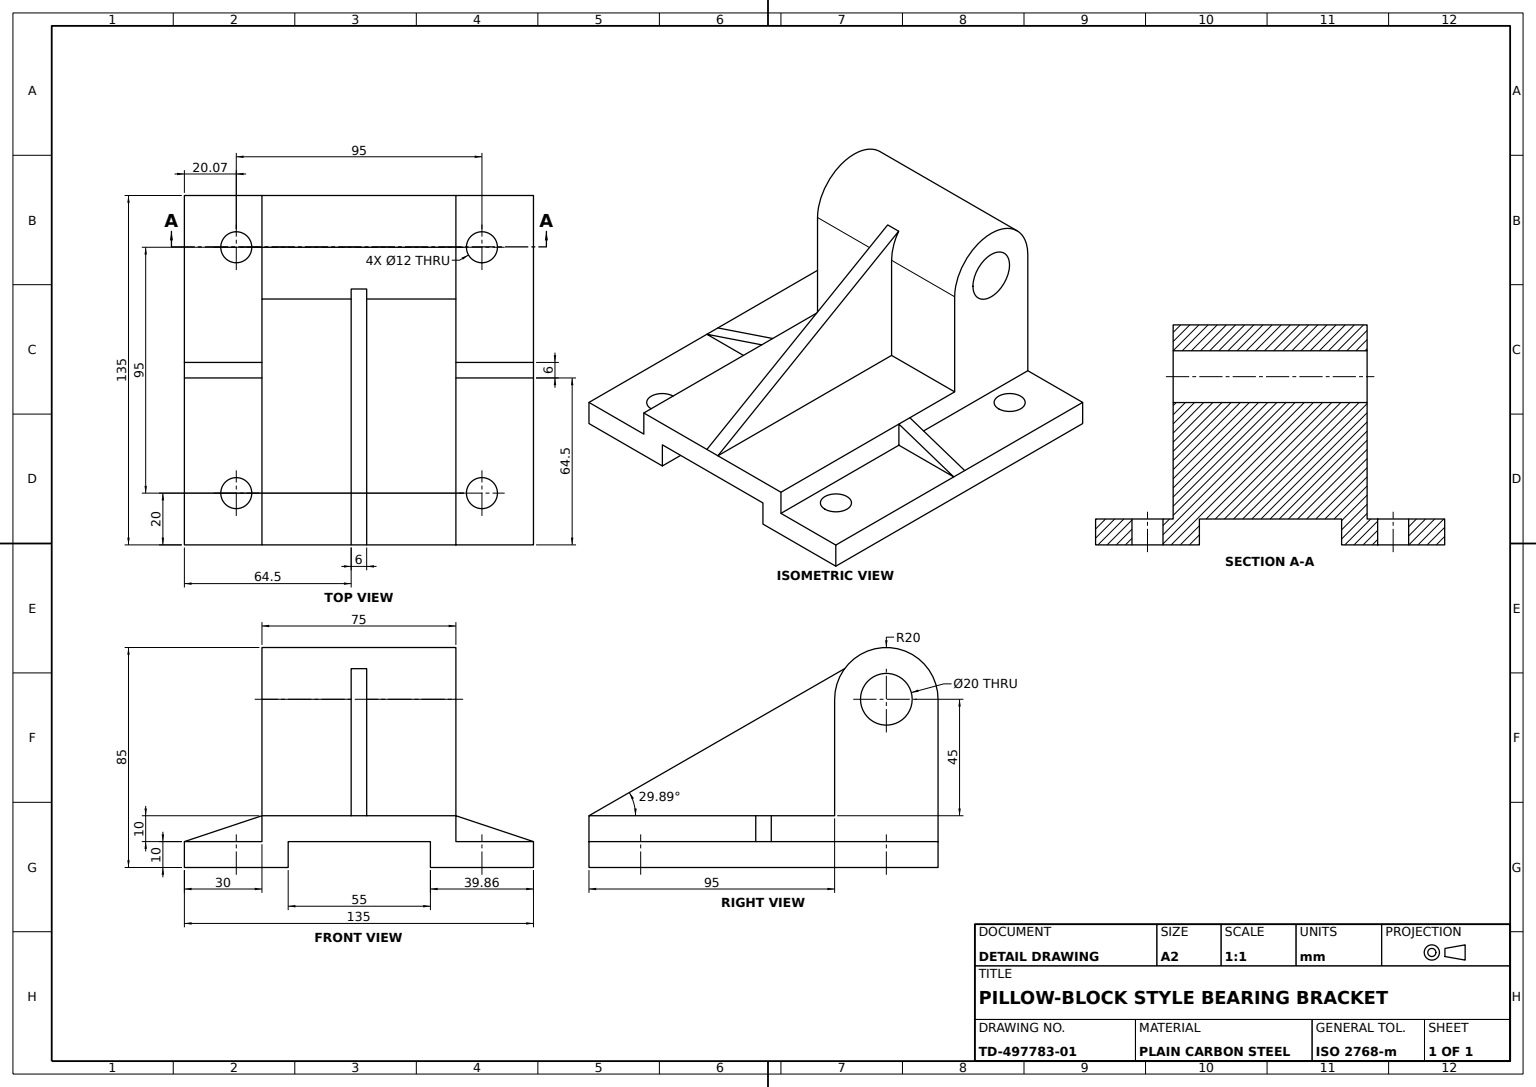
SolidWorks part; units mm, degrees
material "Plain Carbon Steel"
ref_plane "Front Plane" through (0, 0, 0) normal (0, 0, 1) x (1, 0, 0)
ref_plane "Top Plane" through (0, 0, 0) normal (0, 1, 0) x (1, 0, 0)
ref_plane "Right Plane" through (0, 0, 0) normal (1, 0, 0) x (0, 0, -1)
sketch "Base Plate Sketch" plane through (0, 0, 0) normal (0, 0, 1) x (1, 0, 0)
  line L1 (-67.5, 10) -> (67.5, 10)
  line L2 (-67.5, 10) -> (-67.5, -10)
  line L3 (-67.5, -10) -> (67.5, -10)
  line L4 (67.5, 10) -> (67.5, -10)
  line L5 (-67.5, 10) -> (67.5, -10) construction
  line L6 (-67.5, -10) -> (67.5, 10) construction
  point P0 (0, 0)
  dimension "D1" = 20
  dimension "D2" = 135
extrude "Base Plate" add sketch "Base Plate Sketch" along normal mid plane 135
sketch "Bottom Channel Sketch" plane through (0, 0, 67.5) normal (0, 0, 1) x (1, 0, 0)
  line L0 (0, -10) -> (0, 0) construction
  line L1 (-67.5, -10) -> (67.5, -10) construction
  line L2 (27.6432, 0) -> (0, 0)
  line L3 (0, 0) -> (-27.3568, 0)
  line L4 (-27.3568, 0) -> (-27.3568, -10)
  line L5 (-27.3568, -10) -> (27.6432, -10)
  line L6 (27.6432, -10) -> (27.6432, 0)
  line L7 (67.5, -10) -> (67.5, 10) construction
  dimension "D1" = 55
  dimension "D2" = 10
  dimension "D3" = 39.8568
extrude "Bottom Channel" cut sketch "Bottom Channel Sketch" against normal through all
sketch "Top Recess Sketch" plane through (0, 0, 67.5) normal (0, 0, 1) x (1, 0, 0)
  line L0 (0, 10) -> (-37.5, 10)
  line L1 (67.5, 10) -> (-67.5, 10) construction
  line L2 (-37.5, 10) -> (37.5, 10)
  line L3 (-37.5, 10) -> (-37.5, 0)
  line L4 (-37.5, 0) -> (-67.5, 0)
  line L5 (-67.5, 10) -> (-67.5, -10) construction
  line L6 (-67.5, 0) -> (-67.5, 10)
  line L7 (-67.5, 10) -> (-37.5, 10)
  line L8 (37.5, 10) -> (37.5, 0)
  line L9 (37.5, 0) -> (67.5, 0)
  line L10 (67.5, -10) -> (67.5, 10) construction
  line L11 (67.5, 0) -> (67.5, 10)
  line L13 (37.5, 10) -> (67.5, 10)
  line M7 (67.5, -10) -> (67.5, 10)
  line M8 (67.5, 10) -> (-67.5, 10)
  line M9 (-67.5, 10) -> (-67.5, -10)
  dimension "D1" = 75
  dimension "D2" = 37.5
extrude "Top Recess" cut sketch "Top Recess Sketch" against normal through all contours L4 L3 M8 M9 | L8 L9 M7 M8
sketch "Upright Lug Sketch" plane through (37.5, 0, 0) normal (1, 0, 0) x (0, 0, -1)
  line L0 (67.5, 10) -> (67.5, 55)
  line L2 (67.5, 55) -> (47.5, 55) construction
  line L3 (27.5, 55) -> (27.5, 10)
  line L4 (67.5, 10) -> (-67.5, 10) construction
  line L5 (27.5, 10) -> (67.5, 10)
  arc A0 (67.5, 55) -> (27.5, 55) centre (47.5, 55) ccw
  circle A1 centre (47.5, 55) radius 10
  dimension "D4" = 20
  dimension "D1" = 45
  dimension "D2" = 20
extrude "Upright Lug" add sketch "Upright Lug Sketch" against normal blind 75
ref_plane "Gusset Plane" through (0, 0, 0) normal (0, 0, 1) x (1, 0, 0)
sketch "Side Gusset Sketch" plane through (0, 0, 0) normal (0, 0, 1) x (1, 0, 0)
  line L0 (-67.5, 0) -> (-37.5, 10)
  line L1 (-37.5, 10) -> (-37.5, 0) construction
  line L2 (-37.5, 55) -> (-37.5, 10) construction
  line L3 (-37.5, 10) -> (-37.5, 0)
  line L4 (-37.5, 0) -> (-67.5, 0)
  dimension "D1" = 10
extrude "Side Gusset" add sketch "Side Gusset Sketch" along normal mid plane 6
mirror "Side Gusset Mirror" about plane through (0, 0, 0) normal (1, 0, 0) of "Side Gusset"
sketch "Centre Rib Sketch" plane through (37.5, 0, 0) normal (1, 0, 0) x (0, 0, -1)
  line L0 (-67.5, 10) -> (35.5, 69.198)
  line L2 (29.4497, 10) -> (-67.5, 10)
  line L3 (35.5, 69.198) -> (35.5, 10)
  line L4 (35.5, 10) -> (29.4497, 10)
  line L5 (-3, 0) -> (-3, 10) construction
  line L6 (-3, 0) -> (-67.5, 0) construction
  dimension "D1" = 32.4497
  dimension "D2" = 38.5
  dimension "D3" = 69.198
ref_plane "Plane2" through (0, 0, 0) normal (1, 0, 0) x (0, 0, -1)
extrude "Centre Rib" add sketch "Centre Rib Sketch" along normal mid plane 6 from offset 37.5 offset against normal yes
sketch "Mounting Holes Sketch" plane through (0, -10, 0) normal (0, -1, 0) x (1, 0, 0)
  line L0 (27.6432, -67.5) -> (67.5, -67.5) construction
  line L1 (-67.5, 67.5) -> (-27.3568, 67.5) construction
  line L2 (27.6432, 67.5) -> (67.5, 67.5) construction
  line L3 (27.6432, 67.5) -> (67.5, 67.5)
  line L4 (-67.5, 67.5) -> (-27.3568, 67.5)
  line L5 (-47.4284, 67.5) -> (-47.4284, -67.5) construction
  line L6 (-67.5, -67.5) -> (-27.3568, -67.5) construction
  line L7 (47.5716, 67.5) -> (47.5716, -67.5) construction
  circle A0 centre (-47.4284, -47.5) radius 6
  circle A1 centre (47.5716, -47.5) radius 6
  circle A2 centre (-47.4284, 47.5) radius 6
  circle A3 centre (47.5716, 47.5) radius 6
  dimension "D1" = 12
  dimension "D2" = 12
  dimension "D6" = 20
  dimension "D3" = 20
  dimension "D4" = 20
  dimension "D5" = 20
extrude "Mounting Holes Ø12" cut sketch "Mounting Holes Sketch" against normal through all contours A1 | A0 | A2 | A3
